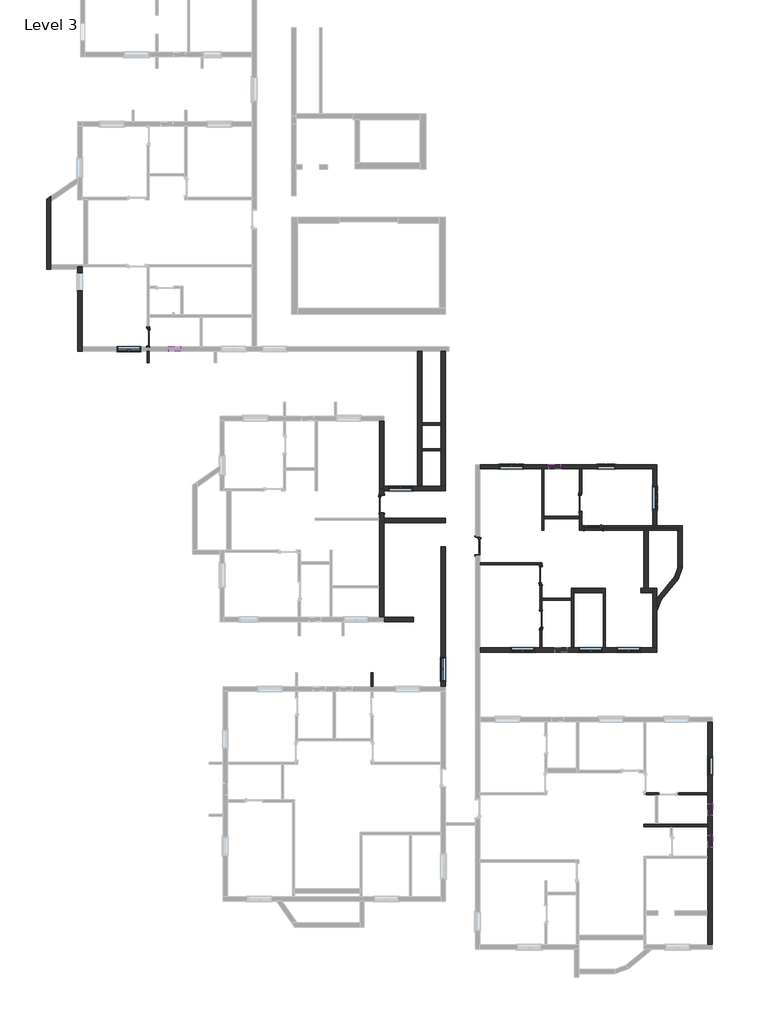
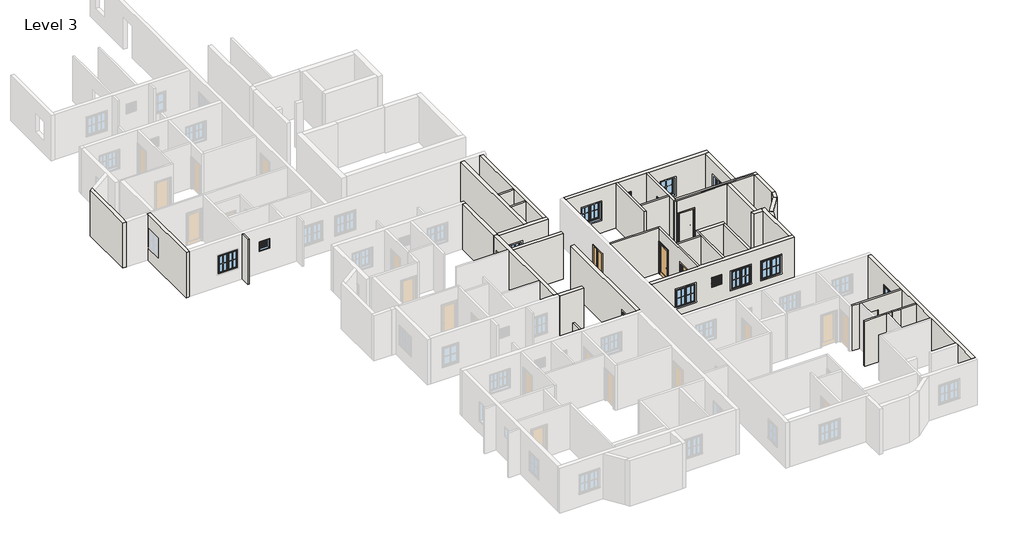
# One storey, part 3 of 7: 39 walls, 15 windows, 7 doors.
"""IFC4 building model written with IfcOpenShell, lengths in millimetres."""

from ifc_helpers import new_model, si_unit, point, frame, frame_2d, origin, place, context, project, spatial, polyline, circle_curve, trimmed, segment, composite_curve, outline, extrude, faceted_brep, transform, mapped, element, save
from components import door_3c6ab76a, door_a3feeac7, door_3b97b8e7, door_868ee8a9, window_272f20d6, window_casement_double_4_x_4_af3140d2, window_f2d8fef0

model = new_model("IFC4")

# Units and contexts
model_context = context("Model", 3, world=origin())
ifc_project = project(units=[si_unit("LENGTHUNIT", "METRE", prefix="MILLI")], contexts=[model_context])

# Site, building, storey
site = spatial("IfcSite", under=ifc_project)
building = spatial("IfcBuilding", under=site)
storey = spatial("IfcBuildingStorey", under=building, Name="Level 3", Elevation=3200.4)

# Doors
placement = place(None, origin())
door_shape = door_3c6ab76a(model_context)
element("IfcDoor", 1, ObjectType="Door-Interior-Single-1_Panel-Wood : 2'6\" x 7' door", at=placement, inside=storey, context=model_context, shape_type="MappedRepresentation", body=[
    mapped(door_shape, transform((-11252.4759469, 2064.0461172, 3200.4), x_axis=(0.0, -1.0, 0.0), y_axis=(1.0, 0.0, 0.0), z_axis=(0.0, 0.0, 1.0))),
])
door_2_shape = door_a3feeac7(model_context)
element("IfcDoor", 2, ObjectType="Door-Interior-Single-1_Panel-Wood : 2'6\" x 7' door", at=placement, inside=storey, context=model_context, shape_type="MappedRepresentation", body=[
    mapped(door_2_shape, transform((11042.3740531, -6465.2997229, 3200.4), x_axis=(0.0, -1.0, 0.0), y_axis=(1.0, 0.0, 0.0), z_axis=(0.0, 0.0, 1.0))),
])
element("IfcDoor", 3, ObjectType="Door-Interior-Single-1_Panel-Wood : 2'6\" x 7' door", at=placement, inside=storey, context=model_context, shape_type="MappedRepresentation", body=[
    mapped(door_2_shape, transform((9004.0240531, -12510.4997229, 3200.4), x_axis=(0.0, 1.0, 0.0), y_axis=(-1.0, 0.0, 0.0), z_axis=(0.0, 0.0, 1.0))),
])
element("IfcDoor", 4, ObjectType="Door-Interior-Single-1_Panel-Wood : 36\" x 84\"", at=placement, inside=storey, context=model_context, shape_type="MappedRepresentation", body=[
    mapped(door_shape, transform((8997.6740531, -10224.4997229, 3200.4), x_axis=(0.0, 1.0, 0.0), y_axis=(-1.0, 0.0, 0.0), z_axis=(0.0, 0.0, 1.0))),
])
door_3_shape = door_3b97b8e7(model_context)
element("IfcDoor", 5, ObjectType="Door-Interior-Single-1_Panel-Wood : 36\" x 84\"", at=placement, inside=storey, context=model_context, shape_type="MappedRepresentation", body=[
    mapped(door_3_shape, transform((5733.7740531, -8700.4997229, 3200.4), x_axis=(0.0, -1.0, 0.0), y_axis=(1.0, 0.0, 0.0), z_axis=(0.0, 0.0, 1.0))),
])
door_4_shape = door_868ee8a9(model_context)
element("IfcDoor", 6, ObjectType="Door-Interior-Single-1_Panel-Wood : 36\" x 84\"", at=placement, inside=storey, context=model_context, shape_type="MappedRepresentation", body=[
    mapped(door_4_shape, transform((787.1240531, -6537.0288828, 3200.4), x_axis=(0.0, -1.0, 0.0), y_axis=(1.0, 0.0, 0.0), z_axis=(0.0, 0.0, 1.0))),
])
element("IfcDoor", 7, ObjectType="Door-Interior-Single-1_Panel-Wood : 36\" x 84\"", at=placement, inside=storey, context=model_context, shape_type="MappedRepresentation", body=[
    mapped(door_4_shape, transform((11712.2990531, -7776.5747229, 3200.4), x_axis=(-1.0, 0.0, 0.0), y_axis=(0.0, -1.0, 0.0), z_axis=(0.0, 0.0, 1.0))),
])

# Walls
element("IfcWall", 8, ObjectType="4.5\" wall", at=placement, inside=storey, context=model_context, shape_type="SweptSolid", body=[
    extrude(outline(polyline([(-11312.8009469, 730.5461172), (-11312.8009469, 1340.1461172), (-11198.5009469, 1340.1461172), (-11198.5009469, 730.5461172), (-11312.8009469, 730.5461172)])), frame((0.0, 0.0, 3200.4), z_axis=(0.0, 0.0, 1.0), x_axis=(1.0, 0.0, 0.0)), (0.0, 0.0, 1.0), 3048.0),
])
element("IfcWall", 9, ObjectType="4.5\" wall", at=placement, inside=storey, context=model_context, shape_type="SweptSolid", body=[
    extrude(outline(polyline([(3850.9990531, -3803.3538828), (2860.3990531, -3803.3538828), (2860.3990531, -3689.0538828), (3850.9990531, -3689.0538828), (3850.9990531, -3803.3538828)])), frame((0.0, 0.0, 3200.4), z_axis=(0.0, 0.0, 1.0), x_axis=(1.0, 0.0, 0.0)), (0.0, 0.0, 1.0), 3048.0),
])
element("IfcWall", 10, ObjectType="4.5\" wall", at=placement, inside=storey, context=model_context, shape_type="SweptSolid", body=[
    extrude(outline(polyline([(2860.3990531, -2355.5538828), (3850.9990531, -2355.5538828), (3850.9990531, -2469.8538828), (2860.3990531, -2469.8538828), (2860.3990531, -2355.5538828)])), frame((0.0, 0.0, 3200.4), z_axis=(0.0, 0.0, 1.0), x_axis=(1.0, 0.0, 0.0)), (0.0, 0.0, 1.0), 3048.0),
])
element("IfcWall", 11, ObjectType="4.5\" wall", at=placement, inside=storey, context=model_context, shape_type="SweptSolid", body=[
    extrude(outline(polyline([(345.7990531, -15233.3538828), (345.7990531, -15957.2538828), (231.4990531, -15957.2538828), (231.4990531, -15233.3538828), (345.7990531, -15233.3538828)])), frame((0.0, 0.0, 3200.4), z_axis=(0.0, 0.0, 1.0), x_axis=(1.0, 0.0, 0.0)), (0.0, 0.0, 1.0), 3048.0),
])
element("IfcWall", 12, ObjectType="4.5\" wall", at=placement, inside=storey, context=model_context, shape_type="Brep", body=[
    faceted_brep([(17617.7990531, -21521.1497229, 6248.4), (15026.9990531, -21521.1497229, 6248.4), (14912.6990531, -21521.1497229, 6248.4), (14417.3990531, -21521.1497229, 6248.4), (14417.3990531, -21521.1497229, 3200.4), (14912.6990531, -21521.1497229, 3200.4), (15026.9990531, -21521.1497229, 3200.4), (15096.8490531, -21521.1497229, 3200.4), (15096.8490531, -21521.1497229, 5359.4), (16062.0490531, -21521.1497229, 5359.4), (16062.0490531, -21521.1497229, 3200.4), (17617.7990531, -21521.1497229, 3200.4), (14417.3990531, -21406.8497229, 6248.4), (17617.7990531, -21406.8497229, 6248.4), (17617.7990531, -21406.8497229, 3200.4), (16062.0490531, -21406.8497229, 3200.4), (16062.0490531, -21406.8497229, 5359.4), (15096.8490531, -21406.8497229, 5359.4), (15096.8490531, -21406.8497229, 3200.4), (14417.3990531, -21406.8497229, 3200.4)], [[[0, 1, 2, 3, 4, 5, 6, 7, 8, 9, 10, 11]], [[12, 13, 14, 15, 16, 17, 18, 19]], [[14, 11, 10, 15]], [[4, 19, 18, 7, 6, 5]], [[3, 2, 1, 0, 13, 12]], [[0, 11, 14, 13]], [[4, 3, 12, 19]], [[17, 8, 7, 18]], [[8, 17, 16, 9]], [[9, 16, 15, 10]]]),
])
element("IfcWall", 13, ObjectType="4.5\" wall", at=placement, inside=storey, context=model_context, shape_type="SweptSolid", body=[
    extrude(outline(polyline([(16055.6990531, -23045.1497229), (16589.0990531, -23045.1497229), (16589.0990531, -23159.4497229), (16055.6990531, -23159.4497229), (16055.6990531, -23045.1497229)])), frame((0.0, 0.0, 3200.4), z_axis=(0.0, 0.0, 1.0), x_axis=(1.0, 0.0, 0.0)), (0.0, 0.0, 1.0), 3048.0),
])
element("IfcWall", 14, ObjectType="4.5\" wall", at=placement, inside=storey, context=model_context, shape_type="Brep", body=[
    faceted_brep([(17617.7990531, -23045.1497229, 3200.4), (15026.9990531, -23045.1497229, 3200.4), (14912.6990531, -23045.1497229, 3200.4), (14303.0990531, -23045.1497229, 3200.4), (14303.0990531, -23045.1497229, 6248.4), (14912.6990531, -23045.1497229, 6248.4), (15026.9990531, -23045.1497229, 6248.4), (17617.7990531, -23045.1497229, 6248.4), (17617.7990531, -23159.4497229, 3200.4), (17617.7990531, -23159.4497229, 6248.4), (15788.9990531, -23159.4497229, 6248.4), (15674.6990531, -23159.4497229, 6248.4), (14303.0990531, -23159.4497229, 6248.4), (14303.0990531, -23159.4497229, 3200.4), (15674.6990531, -23159.4497229, 3200.4), (15788.9990531, -23159.4497229, 3200.4)], [[[0, 1, 2, 3, 4, 5, 6, 7]], [[8, 9, 10, 11, 12, 13, 14, 15]], [[3, 2, 1, 0, 8, 15, 14, 13]], [[4, 3, 13, 12]], [[7, 6, 5, 4, 12, 11, 10, 9]], [[0, 7, 9, 8]]]),
])
element("IfcWall", 15, ObjectType="4.5\" wall", at=placement, inside=storey, context=model_context, shape_type="Brep", body=[
    faceted_brep([(10988.3990531, -7894.0497229, 3200.4), (14303.0990531, -7894.0497229, 3200.4), (14531.6990531, -7894.0497229, 3200.4), (16055.6990531, -7894.0497229, 3200.4), (16055.6990531, -7894.0497229, 6248.4), (14531.6990531, -7894.0497229, 6248.4), (14303.0990531, -7894.0497229, 6248.4), (10988.3990531, -7894.0497229, 6248.4), (10988.3990531, -7779.7497229, 3200.4), (10988.3990531, -7779.7497229, 6248.4), (11102.6990531, -7779.7497229, 6248.4), (14760.2990531, -7779.7497229, 6248.4), (14988.8990531, -7779.7497229, 6248.4), (16055.6990531, -7779.7497229, 6248.4), (16055.6990531, -7779.7497229, 3200.4), (14988.8990531, -7779.7497229, 3200.4), (14760.2990531, -7779.7497229, 3200.4), (11102.6990531, -7779.7497229, 3200.4)], [[[0, 1, 2, 3, 4, 5, 6, 7]], [[8, 9, 10, 11, 12, 13, 14, 15, 16, 17]], [[3, 2, 1, 0, 8, 17, 16, 15, 14]], [[7, 6, 5, 4, 13, 12, 11, 10, 9]], [[0, 7, 9, 8]], [[4, 3, 14, 13]]]),
])
element("IfcWall", 16, ObjectType="4.5\" wall", at=placement, inside=storey, context=model_context, shape_type="Brep", body=[
    faceted_brep([(10696.2990531, -13939.2497229, 3200.4), (10696.2990531, -11119.8497229, 3200.4), (10696.2990531, -10891.2497229, 3200.4), (10696.2990531, -10891.2497229, 6248.4), (10696.2990531, -11119.8497229, 6248.4), (10696.2990531, -13939.2497229, 6248.4), (10581.9990531, -13939.2497229, 3200.4), (10581.9990531, -13939.2497229, 6248.4), (10581.9990531, -11500.8497229, 6248.4), (10581.9990531, -11386.5497229, 6248.4), (10581.9990531, -10891.2497229, 6248.4), (10581.9990531, -10891.2497229, 3200.4), (10581.9990531, -11386.5497229, 3200.4), (10581.9990531, -11500.8497229, 3200.4)], [[[0, 1, 2, 3, 4, 5]], [[6, 7, 8, 9, 10, 11, 12, 13]], [[2, 1, 0, 6, 13, 12, 11]], [[5, 4, 3, 10, 9, 8, 7]], [[0, 5, 7, 6]], [[3, 2, 11, 10]]]),
])
element("IfcWall", 17, ObjectType="4.5\" wall", at=placement, inside=storey, context=model_context, shape_type="SweptSolid", body=[
    extrude(outline(polyline([(9057.9990531, -11386.5497229), (10581.9990531, -11386.5497229), (10581.9990531, -11500.8497229), (9057.9990531, -11500.8497229), (9057.9990531, -11386.5497229)])), frame((0.0, 0.0, 3200.4), z_axis=(0.0, 0.0, 1.0), x_axis=(1.0, 0.0, 0.0)), (0.0, 0.0, 1.0), 3048.0),
])
element("IfcWall", 18, ObjectType="4.5\" wall", at=placement, inside=storey, context=model_context, shape_type="Brep", body=[
    faceted_brep([(8943.6990531, -13939.2497229, 6248.4), (8943.6990531, -9672.0497229, 6248.4), (8943.6990531, -9557.7497229, 6248.4), (8943.6990531, -9557.7497229, 3200.4), (8943.6990531, -9672.0497229, 3200.4), (8943.6990531, -9741.8997229, 3200.4), (8943.6990531, -9741.8997229, 5359.4), (8943.6990531, -10707.0997229, 5359.4), (8943.6990531, -10707.0997229, 3200.4), (8943.6990531, -12027.8997229, 3200.4), (8943.6990531, -12027.8997229, 5359.4), (8943.6990531, -12993.0997229, 5359.4), (8943.6990531, -12993.0997229, 3200.4), (8943.6990531, -13939.2497229, 3200.4), (9057.9990531, -9557.7497229, 6248.4), (9057.9990531, -11386.5497229, 6248.4), (9057.9990531, -11500.8497229, 6248.4), (9057.9990531, -13939.2497229, 6248.4), (9057.9990531, -13939.2497229, 3200.4), (9057.9990531, -12993.0997229, 3200.4), (9057.9990531, -12993.0997229, 5359.4), (9057.9990531, -12027.8997229, 5359.4), (9057.9990531, -12027.8997229, 3200.4), (9057.9990531, -11500.8497229, 3200.4), (9057.9990531, -11386.5497229, 3200.4), (9057.9990531, -10707.0997229, 3200.4), (9057.9990531, -10707.0997229, 5359.4), (9057.9990531, -9741.8997229, 5359.4), (9057.9990531, -9741.8997229, 3200.4), (9057.9990531, -9557.7497229, 3200.4)], [[[0, 1, 2, 3, 4, 5, 6, 7, 8, 9, 10, 11, 12, 13]], [[14, 15, 16, 17, 18, 19, 20, 21, 22, 23, 24, 25, 26, 27, 28, 29]], [[18, 13, 12, 19]], [[3, 29, 28, 5, 4]], [[22, 9, 8, 25, 24, 23]], [[2, 1, 0, 17, 16, 15, 14]], [[0, 13, 18, 17]], [[3, 2, 14, 29]], [[21, 10, 9, 22]], [[10, 21, 20, 11]], [[11, 20, 19, 12]], [[27, 6, 5, 28]], [[6, 27, 26, 7]], [[7, 26, 25, 8]]]),
])
element("IfcWall", 19, ObjectType="4.5\" wall", at=placement, inside=storey, context=model_context, shape_type="SweptSolid", body=[
    extrude(outline(polyline([(8943.6990531, -9672.0497229), (5844.8990531, -9672.0497229), (5844.8990531, -9557.7497229), (8943.6990531, -9557.7497229), (8943.6990531, -9672.0497229)])), frame((0.0, 0.0, 3200.4), z_axis=(0.0, 0.0, 1.0), x_axis=(1.0, 0.0, 0.0)), (0.0, 0.0, 1.0), 3048.0),
])
element("IfcWall", 20, ObjectType="4.5\" wall", at=placement, inside=storey, context=model_context, shape_type="Brep", body=[
    faceted_brep([(9045.2990531, -4731.7497229, 3200.4), (9045.2990531, -7894.0497229, 3200.4), (9045.2990531, -7894.0497229, 6248.4), (9045.2990531, -4731.7497229, 6248.4), (9159.5990531, -4731.7497229, 3200.4), (9159.5990531, -4731.7497229, 6248.4), (9159.5990531, -7170.1497229, 6248.4), (9159.5990531, -7284.4497229, 6248.4), (9159.5990531, -7894.0497229, 6248.4), (9159.5990531, -7894.0497229, 3200.4), (9159.5990531, -7284.4497229, 3200.4), (9159.5990531, -7170.1497229, 3200.4)], [[[0, 1, 2, 3]], [[4, 5, 6, 7, 8, 9, 10, 11]], [[1, 0, 4, 11, 10, 9]], [[2, 1, 9, 8]], [[3, 2, 8, 7, 6, 5]], [[0, 3, 5, 4]]]),
])
element("IfcWall", 21, ObjectType="4.5\" wall", at=placement, inside=storey, context=model_context, shape_type="Brep", body=[
    faceted_brep([(10988.3990531, -7779.7497229, 6248.4), (10988.3990531, -7284.4497229, 6248.4), (10988.3990531, -7170.1497229, 6248.4), (10988.3990531, -4731.7497229, 6248.4), (10988.3990531, -4731.7497229, 3200.4), (10988.3990531, -5982.6997229, 3200.4), (10988.3990531, -5982.6997229, 5359.4), (10988.3990531, -6947.8997229, 5359.4), (10988.3990531, -6947.8997229, 3200.4), (10988.3990531, -7170.1497229, 3200.4), (10988.3990531, -7284.4497229, 3200.4), (10988.3990531, -7779.7497229, 3200.4), (11102.6990531, -4731.7497229, 6248.4), (11102.6990531, -7665.4497229, 6248.4), (11102.6990531, -7779.7497229, 6248.4), (11102.6990531, -7779.7497229, 3200.4), (11102.6990531, -7665.4497229, 3200.4), (11102.6990531, -6947.8997229, 3200.4), (11102.6990531, -6947.8997229, 5359.4), (11102.6990531, -5982.6997229, 5359.4), (11102.6990531, -5982.6997229, 3200.4), (11102.6990531, -4731.7497229, 3200.4)], [[[0, 1, 2, 3, 4, 5, 6, 7, 8, 9, 10, 11]], [[12, 13, 14, 15, 16, 17, 18, 19, 20, 21]], [[4, 21, 20, 5]], [[15, 11, 10, 9, 8, 17, 16]], [[3, 2, 1, 0, 14, 13, 12]], [[4, 3, 12, 21]], [[0, 11, 15, 14]], [[7, 18, 17, 8]], [[18, 7, 6, 19]], [[19, 6, 5, 20]]]),
])
element("IfcWall", 22, ObjectType="4.5\" wall", at=placement, inside=storey, context=model_context, shape_type="SweptSolid", body=[
    extrude(outline(polyline([(10988.3990531, -7284.4497229), (9159.5990531, -7284.4497229), (9159.5990531, -7170.1497229), (10988.3990531, -7170.1497229), (10988.3990531, -7284.4497229)])), frame((0.0, 0.0, 3200.4), z_axis=(0.0, 0.0, 1.0), x_axis=(1.0, 0.0, 0.0)), (0.0, 0.0, 1.0), 3048.0),
])
element("IfcWall", 23, ObjectType="4.5\" wall", at=placement, inside=storey, context=model_context, shape_type="SweptSolid", body=[
    extrude(outline(polyline([(12220.2990531, -13939.2497229), (12220.2990531, -11119.8497229), (12334.5990531, -11119.8497229), (12334.5990531, -13939.2497229), (12220.2990531, -13939.2497229)])), frame((0.0, 0.0, 3200.4), z_axis=(0.0, 0.0, 1.0), x_axis=(1.0, 0.0, 0.0)), (0.0, 0.0, 1.0), 3048.0),
])
element("IfcWall", 24, ObjectType="9\"", at=placement, inside=storey, context=model_context, shape_type="Brep", body=[
    faceted_brep([(-14894.2009469, 5683.5461172, 3200.4), (-14894.2009469, 5569.2461172, 3200.4), (-14894.2009469, 1340.1461172, 3200.4), (-14894.2009469, 1340.1461172, 6248.4), (-14894.2009469, 5569.2461172, 6248.4), (-14894.2009469, 5683.5461172, 6248.4), (-14894.2009469, 5378.7461172, 5334.0), (-14894.2009469, 4464.3461172, 5334.0), (-14894.2009469, 4464.3461172, 4114.8), (-14894.2009469, 5378.7461172, 4114.8), (-14665.6009469, 5683.5461172, 3200.4), (-14665.6009469, 5683.5461172, 6248.4), (-14665.6009469, 1568.7461172, 6248.4), (-14665.6009469, 1340.1461172, 6248.4), (-14665.6009469, 1340.1461172, 3200.4), (-14665.6009469, 1568.7461172, 3200.4), (-14665.6009469, 5378.7461172, 5334.0), (-14665.6009469, 5378.7461172, 4114.8), (-14665.6009469, 4464.3461172, 4114.8), (-14665.6009469, 4464.3461172, 5334.0)], [[[0, 1, 2, 3, 4, 5], [6, 7, 8, 9]], [[10, 11, 12, 13, 14, 15], [16, 17, 18, 19]], [[2, 1, 0, 10, 15, 14]], [[5, 4, 3, 13, 12, 11]], [[3, 2, 14, 13]], [[0, 5, 11, 10]], [[17, 16, 6, 9]], [[18, 17, 9, 8]], [[19, 18, 8, 7]], [[16, 19, 7, 6]]]),
])
element("IfcWall", 25, ObjectType="9\"", at=placement, inside=storey, context=model_context, shape_type="Brep", body=[
    faceted_brep([(904.5990531, -5746.4538828, 3200.4), (904.5990531, -5632.1538828, 3200.4), (904.5990531, -2241.2538828, 3200.4), (904.5990531, -2241.2538828, 6248.4), (904.5990531, -5632.1538828, 6248.4), (904.5990531, -5746.4538828, 6248.4), (675.9990531, -5746.4538828, 3200.4), (675.9990531, -5746.4538828, 6248.4), (675.9990531, -2241.2538828, 6248.4), (675.9990531, -2241.2538828, 3200.4)], [[[0, 1, 2, 3, 4, 5]], [[6, 7, 8, 9]], [[2, 1, 0, 6, 9]], [[5, 4, 3, 8, 7]], [[0, 5, 7, 6]], [[3, 2, 9, 8]]]),
])
element("IfcWall", 26, ObjectType="9\"", at=placement, inside=storey, context=model_context, shape_type="Brep", body=[
    faceted_brep([(904.5990531, -5746.4538828, 3200.4), (904.5990531, -5746.4538828, 6248.4), (904.5990531, -5860.7538828, 6248.4), (904.5990531, -7270.4538828, 6248.4), (904.5990531, -7499.0538828, 6248.4), (904.5990531, -12375.8538828, 6248.4), (904.5990531, -12375.8538828, 3200.4), (904.5990531, -7499.0538828, 3200.4), (904.5990531, -7270.4538828, 3200.4), (904.5990531, -7019.6288828, 3200.4), (904.5990531, -7019.6288828, 5359.4), (904.5990531, -6054.4288828, 5359.4), (904.5990531, -6054.4288828, 3200.4), (904.5990531, -5860.7538828, 3200.4), (675.9990531, -5746.4538828, 6248.4), (675.9990531, -5746.4538828, 3200.4), (675.9990531, -6054.4288828, 3200.4), (675.9990531, -6054.4288828, 5359.4), (675.9990531, -7019.6288828, 5359.4), (675.9990531, -7019.6288828, 3200.4), (675.9990531, -7270.4538828, 3200.4), (675.9990531, -7384.7538828, 3200.4), (675.9990531, -10737.5538828, 3200.4), (675.9990531, -10851.8538828, 3200.4), (675.9990531, -12375.8538828, 3200.4), (675.9990531, -12375.8538828, 6248.4), (675.9990531, -10851.8538828, 6248.4), (675.9990531, -10737.5538828, 6248.4), (675.9990531, -7384.7538828, 6248.4), (675.9990531, -7270.4538828, 6248.4)], [[[0, 1, 2, 3, 4, 5, 6, 7, 8, 9, 10, 11, 12, 13]], [[14, 15, 16, 17, 18, 19, 20, 21, 22, 23, 24, 25, 26, 27, 28, 29]], [[6, 24, 23, 22, 21, 20, 19, 9, 8, 7]], [[15, 0, 13, 12, 16]], [[1, 0, 15, 14]], [[5, 4, 3, 2, 1, 14, 29, 28, 27, 26, 25]], [[6, 5, 25, 24]], [[18, 10, 9, 19]], [[10, 18, 17, 11]], [[11, 17, 16, 12]]]),
])
element("IfcWall", 27, ObjectType="9\"", at=placement, inside=storey, context=model_context, shape_type="SweptSolid", body=[
    extrude(outline(polyline([(904.5990531, -7270.4538828), (4079.5990531, -7270.4538828), (4079.5990531, -7499.0538828), (904.5990531, -7499.0538828), (904.5990531, -7270.4538828)])), frame((0.0, 0.0, 3200.4), z_axis=(0.0, 0.0, 1.0), x_axis=(1.0, 0.0, 0.0)), (0.0, 0.0, 1.0), 3048.0),
])
element("IfcWall", 28, ObjectType="9\"", at=placement, inside=storey, context=model_context, shape_type="Brep", body=[
    faceted_brep([(904.5990531, -5860.7538828, 3200.4), (4079.5990531, -5860.7538828, 3200.4), (4079.5990531, -5860.7538828, 6248.4), (904.5990531, -5860.7538828, 6248.4), (2377.7990531, -5860.7538828, 5334.0), (2377.7990531, -5860.7538828, 4114.8), (1158.5990531, -5860.7538828, 4114.8), (1158.5990531, -5860.7538828, 5334.0), (904.5990531, -5632.1538828, 3200.4), (904.5990531, -5632.1538828, 6248.4), (2631.7990531, -5632.1538828, 6248.4), (2860.3990531, -5632.1538828, 6248.4), (3850.9990531, -5632.1538828, 6248.4), (4079.5990531, -5632.1538828, 6248.4), (4079.5990531, -5632.1538828, 3200.4), (3850.9990531, -5632.1538828, 3200.4), (2860.3990531, -5632.1538828, 3200.4), (2631.7990531, -5632.1538828, 3200.4), (2377.7990531, -5632.1538828, 5334.0), (1158.5990531, -5632.1538828, 5334.0), (1158.5990531, -5632.1538828, 4114.8), (2377.7990531, -5632.1538828, 4114.8), (904.5990531, -5746.4538828, 3200.4), (904.5990531, -5746.4538828, 6248.4)], [[[0, 1, 2, 3], [4, 5, 6, 7]], [[8, 9, 10, 11, 12, 13, 14, 15, 16, 17], [18, 19, 20, 21]], [[1, 0, 22, 8, 17, 16, 15, 14]], [[3, 2, 13, 12, 11, 10, 9, 23]], [[0, 3, 23, 9, 8, 22]], [[2, 1, 14, 13]], [[5, 4, 18, 21]], [[6, 5, 21, 20]], [[7, 6, 20, 19]], [[4, 7, 19, 18]]]),
])
element("IfcWall", 29, ObjectType="9\"", at=placement, inside=storey, context=model_context, shape_type="Brep", body=[
    faceted_brep([(2631.7990531, 1340.1461172, 3200.4), (2631.7990531, -5632.1538828, 3200.4), (2631.7990531, -5632.1538828, 6248.4), (2631.7990531, 1340.1461172, 6248.4), (2860.3990531, 1340.1461172, 3200.4), (2860.3990531, 1340.1461172, 6248.4), (2860.3990531, -2355.5538828, 6248.4), (2860.3990531, -2469.8538828, 6248.4), (2860.3990531, -3689.0538828, 6248.4), (2860.3990531, -3803.3538828, 6248.4), (2860.3990531, -5632.1538828, 6248.4), (2860.3990531, -5632.1538828, 3200.4), (2860.3990531, -3803.3538828, 3200.4), (2860.3990531, -3689.0538828, 3200.4), (2860.3990531, -2469.8538828, 3200.4), (2860.3990531, -2355.5538828, 3200.4)], [[[0, 1, 2, 3]], [[4, 5, 6, 7, 8, 9, 10, 11, 12, 13, 14, 15]], [[1, 0, 4, 15, 14, 13, 12, 11]], [[3, 2, 10, 9, 8, 7, 6, 5]], [[0, 3, 5, 4]], [[2, 1, 11, 10]]]),
])
element("IfcWall", 30, ObjectType="9\"", at=placement, inside=storey, context=model_context, shape_type="Brep", body=[
    faceted_brep([(4079.5990531, -5632.1538828, 3200.4), (4079.5990531, 1340.1461172, 3200.4), (4079.5990531, 1340.1461172, 6248.4), (4079.5990531, -5632.1538828, 6248.4), (3850.9990531, -5632.1538828, 3200.4), (3850.9990531, -5632.1538828, 6248.4), (3850.9990531, -3803.3538828, 6248.4), (3850.9990531, -3689.0538828, 6248.4), (3850.9990531, -2469.8538828, 6248.4), (3850.9990531, -2355.5538828, 6248.4), (3850.9990531, 1340.1461172, 6248.4), (3850.9990531, 1340.1461172, 3200.4), (3850.9990531, -2355.5538828, 3200.4), (3850.9990531, -2469.8538828, 3200.4), (3850.9990531, -3689.0538828, 3200.4), (3850.9990531, -3803.3538828, 3200.4)], [[[0, 1, 2, 3]], [[4, 5, 6, 7, 8, 9, 10, 11, 12, 13, 14, 15]], [[1, 0, 4, 15, 14, 13, 12, 11]], [[3, 2, 10, 9, 8, 7, 6, 5]], [[2, 1, 11, 10]], [[0, 3, 5, 4]]]),
])
element("IfcWall", 31, ObjectType="9\"", at=placement, inside=storey, context=model_context, shape_type="SweptSolid", body=[
    extrude(outline(polyline([(904.5990531, -12375.8538828), (2441.2990531, -12375.8538828), (2441.2990531, -12604.4538828), (904.5990531, -12604.4538828), (904.5990531, -12375.8538828)])), frame((0.0, 0.0, 3200.4), z_axis=(0.0, 0.0, 1.0), x_axis=(1.0, 0.0, 0.0)), (0.0, 0.0, 1.0), 3048.0),
])
element("IfcWall", 32, ObjectType="9\"", at=placement, inside=storey, context=model_context, shape_type="Brep", body=[
    faceted_brep([(17617.7990531, -17749.2497229, 3200.4), (17617.7990531, -21406.8497229, 3200.4), (17617.7990531, -21521.1497229, 3200.4), (17617.7990531, -23045.1497229, 3200.4), (17617.7990531, -23159.4497229, 3200.4), (17617.7990531, -24683.4497229, 3200.4), (17617.7990531, -24797.7497229, 3200.4), (17617.7990531, -27502.8497229, 3200.4), (17617.7990531, -27731.4497229, 3200.4), (17617.7990531, -29255.4497229, 3200.4), (17617.7990531, -29255.4497229, 6248.4), (17617.7990531, -27731.4497229, 6248.4), (17617.7990531, -27502.8497229, 6248.4), (17617.7990531, -24797.7497229, 6248.4), (17617.7990531, -24683.4497229, 6248.4), (17617.7990531, -23159.4497229, 6248.4), (17617.7990531, -23045.1497229, 6248.4), (17617.7990531, -21521.1497229, 6248.4), (17617.7990531, -21406.8497229, 6248.4), (17617.7990531, -17749.2497229, 6248.4), (17617.7990531, -22587.9497229, 5334.0), (17617.7990531, -22587.9497229, 4724.4), (17617.7990531, -21978.3497229, 4724.4), (17617.7990531, -21978.3497229, 5334.0), (17617.7990531, -23616.6497229, 5334.0), (17617.7990531, -24226.2497229, 5334.0), (17617.7990531, -24226.2497229, 4724.4), (17617.7990531, -23616.6497229, 4724.4), (17617.7990531, -19584.3997229, 5334.0), (17617.7990531, -20498.7997229, 5334.0), (17617.7990531, -20498.7997229, 4114.8), (17617.7990531, -19584.3997229, 4114.8), (17846.3990531, -17749.2497229, 3200.4), (17846.3990531, -17749.2497229, 6248.4), (17846.3990531, -29255.4497229, 6248.4), (17846.3990531, -29255.4497229, 3200.4), (17846.3990531, -22587.9497229, 5334.0), (17846.3990531, -21978.3497229, 5334.0), (17846.3990531, -21978.3497229, 4724.4), (17846.3990531, -22587.9497229, 4724.4), (17846.3990531, -23616.6497229, 5334.0), (17846.3990531, -23616.6497229, 4724.4), (17846.3990531, -24226.2497229, 4724.4), (17846.3990531, -24226.2497229, 5334.0), (17846.3990531, -19584.3997229, 5334.0), (17846.3990531, -19584.3997229, 4114.8), (17846.3990531, -20498.7997229, 4114.8), (17846.3990531, -20498.7997229, 5334.0)], [[[0, 1, 2, 3, 4, 5, 6, 7, 8, 9, 10, 11, 12, 13, 14, 15, 16, 17, 18, 19], [20, 21, 22, 23], [24, 25, 26, 27], [28, 29, 30, 31]], [[32, 33, 34, 35], [36, 37, 38, 39], [40, 41, 42, 43], [44, 45, 46, 47]], [[9, 8, 7, 6, 5, 4, 3, 2, 1, 0, 32, 35]], [[19, 18, 17, 16, 15, 14, 13, 12, 11, 10, 34, 33]], [[0, 19, 33, 32]], [[10, 9, 35, 34]], [[21, 20, 36, 39]], [[22, 21, 39, 38]], [[23, 22, 38, 37]], [[20, 23, 37, 36]], [[41, 40, 24, 27]], [[42, 41, 27, 26]], [[43, 42, 26, 25]], [[40, 43, 25, 24]], [[45, 44, 28, 31]], [[46, 45, 31, 30]], [[47, 46, 30, 29]], [[44, 47, 29, 28]]]),
])
element("IfcWall", 33, ObjectType="9\"", at=placement, inside=storey, context=model_context, shape_type="Brep", body=[
    faceted_brep([(5844.8990531, -14167.8497229, 3200.4), (14988.8990531, -14167.8497229, 3200.4), (14988.8990531, -14167.8497229, 6248.4), (5844.8990531, -14167.8497229, 6248.4), (10334.3490531, -14167.8497229, 5334.0), (10334.3490531, -14167.8497229, 4724.4), (9724.7490531, -14167.8497229, 4724.4), (9724.7490531, -14167.8497229, 5334.0), (12912.4490531, -14167.8497229, 5334.0), (14131.6490531, -14167.8497229, 5334.0), (14131.6490531, -14167.8497229, 4114.8), (12912.4490531, -14167.8497229, 4114.8), (10956.6490531, -14167.8497229, 5334.0), (12175.8490531, -14167.8497229, 5334.0), (12175.8490531, -14167.8497229, 4114.8), (10956.6490531, -14167.8497229, 4114.8), (7451.4490531, -14167.8497229, 5334.0), (8670.6490531, -14167.8497229, 5334.0), (8670.6490531, -14167.8497229, 4114.8), (7451.4490531, -14167.8497229, 4114.8), (5844.8990531, -13939.2497229, 3200.4), (5844.8990531, -13939.2497229, 6248.4), (8943.6990531, -13939.2497229, 6248.4), (9057.9990531, -13939.2497229, 6248.4), (10581.9990531, -13939.2497229, 6248.4), (10696.2990531, -13939.2497229, 6248.4), (12220.2990531, -13939.2497229, 6248.4), (12334.5990531, -13939.2497229, 6248.4), (14760.2990531, -13939.2497229, 6248.4), (14988.8990531, -13939.2497229, 6248.4), (14988.8990531, -13939.2497229, 3200.4), (14760.2990531, -13939.2497229, 3200.4), (12334.5990531, -13939.2497229, 3200.4), (12220.2990531, -13939.2497229, 3200.4), (10696.2990531, -13939.2497229, 3200.4), (10581.9990531, -13939.2497229, 3200.4), (9057.9990531, -13939.2497229, 3200.4), (8943.6990531, -13939.2497229, 3200.4), (10334.3490531, -13939.2497229, 5334.0), (9724.7490531, -13939.2497229, 5334.0), (9724.7490531, -13939.2497229, 4724.4), (10334.3490531, -13939.2497229, 4724.4), (12912.4490531, -13939.2497229, 5334.0), (12912.4490531, -13939.2497229, 4114.8), (14131.6490531, -13939.2497229, 4114.8), (14131.6490531, -13939.2497229, 5334.0), (10956.6490531, -13939.2497229, 5334.0), (10956.6490531, -13939.2497229, 4114.8), (12175.8490531, -13939.2497229, 4114.8), (12175.8490531, -13939.2497229, 5334.0), (7451.4490531, -13939.2497229, 5334.0), (7451.4490531, -13939.2497229, 4114.8), (8670.6490531, -13939.2497229, 4114.8), (8670.6490531, -13939.2497229, 5334.0)], [[[0, 1, 2, 3], [4, 5, 6, 7], [8, 9, 10, 11], [12, 13, 14, 15], [16, 17, 18, 19]], [[20, 21, 22, 23, 24, 25, 26, 27, 28, 29, 30, 31, 32, 33, 34, 35, 36, 37], [38, 39, 40, 41], [42, 43, 44, 45], [46, 47, 48, 49], [50, 51, 52, 53]], [[1, 0, 20, 37, 36, 35, 34, 33, 32, 31, 30]], [[3, 2, 29, 28, 27, 26, 25, 24, 23, 22, 21]], [[0, 3, 21, 20]], [[2, 1, 30, 29]], [[5, 4, 38, 41]], [[6, 5, 41, 40]], [[7, 6, 40, 39]], [[4, 7, 39, 38]], [[43, 42, 8, 11]], [[44, 43, 11, 10]], [[45, 44, 10, 9]], [[42, 45, 9, 8]], [[47, 46, 12, 15]], [[48, 47, 15, 14]], [[49, 48, 14, 13]], [[46, 49, 13, 12]], [[51, 50, 16, 19]], [[52, 51, 19, 18]], [[53, 52, 18, 17]], [[50, 53, 17, 16]]]),
])
element("IfcWall", 34, ObjectType="9\"", at=placement, inside=storey, context=model_context, shape_type="SweptSolid", body=[
    extrude(outline(polyline([(-15957.2538828, 3200.4), (-15957.2538828, 6248.4), (-8732.9659091, 6248.4), (-8732.9659091, 3200.4), (-15957.2538828, 3200.4)]), holes=[polyline([(-14445.9538828, 5334.0), (-15665.1538828, 5334.0), (-15665.1538828, 4114.8), (-14445.9538828, 4114.8), (-14445.9538828, 5334.0)])]), frame((3850.9990531, 0.0, 0.0), z_axis=(1.0, 0.0, 0.0), x_axis=(0.0, 1.0, 0.0)), (0.0, 0.0, 1.0), 228.6),
])
element("IfcWall", 35, ObjectType="9\"", at=placement, inside=storey, context=model_context, shape_type="Brep", body=[
    faceted_brep([(5844.8990531, -4731.7497229, 3200.4), (9045.2990531, -4731.7497229, 3200.4), (9159.5990531, -4731.7497229, 3200.4), (10988.3990531, -4731.7497229, 3200.4), (11102.6990531, -4731.7497229, 3200.4), (14760.2990531, -4731.7497229, 3200.4), (14988.8990531, -4731.7497229, 3200.4), (14988.8990531, -4731.7497229, 6248.4), (14760.2990531, -4731.7497229, 6248.4), (11102.6990531, -4731.7497229, 6248.4), (10988.3990531, -4731.7497229, 6248.4), (9159.5990531, -4731.7497229, 6248.4), (9045.2990531, -4731.7497229, 6248.4), (5844.8990531, -4731.7497229, 6248.4), (10016.8490531, -4731.7497229, 5334.0), (10016.8490531, -4731.7497229, 4724.4), (9407.2490531, -4731.7497229, 4724.4), (9407.2490531, -4731.7497229, 5334.0), (12823.5490531, -4731.7497229, 5334.0), (12823.5490531, -4731.7497229, 4114.8), (11909.1490531, -4731.7497229, 4114.8), (11909.1490531, -4731.7497229, 5334.0), (8086.4490531, -4731.7497229, 5334.0), (8086.4490531, -4731.7497229, 4114.8), (6867.2490531, -4731.7497229, 4114.8), (6867.2490531, -4731.7497229, 5334.0), (5844.8990531, -4503.1497229, 3200.4), (5844.8990531, -4503.1497229, 6248.4), (14988.8990531, -4503.1497229, 6248.4), (14988.8990531, -4503.1497229, 3200.4), (10016.8490531, -4503.1497229, 5334.0), (9407.2490531, -4503.1497229, 5334.0), (9407.2490531, -4503.1497229, 4724.4), (10016.8490531, -4503.1497229, 4724.4), (12823.5490531, -4503.1497229, 5334.0), (11909.1490531, -4503.1497229, 5334.0), (11909.1490531, -4503.1497229, 4114.8), (12823.5490531, -4503.1497229, 4114.8), (8086.4490531, -4503.1497229, 5334.0), (6867.2490531, -4503.1497229, 5334.0), (6867.2490531, -4503.1497229, 4114.8), (8086.4490531, -4503.1497229, 4114.8)], [[[0, 1, 2, 3, 4, 5, 6, 7, 8, 9, 10, 11, 12, 13], [14, 15, 16, 17], [18, 19, 20, 21], [22, 23, 24, 25]], [[26, 27, 28, 29], [30, 31, 32, 33], [34, 35, 36, 37], [38, 39, 40, 41]], [[6, 5, 4, 3, 2, 1, 0, 26, 29]], [[13, 12, 11, 10, 9, 8, 7, 28, 27]], [[7, 6, 29, 28]], [[0, 13, 27, 26]], [[15, 14, 30, 33]], [[16, 15, 33, 32]], [[17, 16, 32, 31]], [[14, 17, 31, 30]], [[19, 18, 34, 37]], [[20, 19, 37, 36]], [[21, 20, 36, 35]], [[18, 21, 35, 34]], [[23, 22, 38, 41]], [[24, 23, 41, 40]], [[25, 24, 40, 39]], [[22, 25, 39, 38]]]),
])
element("IfcWall", 36, ObjectType="9\"", at=placement, inside=storey, context=model_context, shape_type="SweptSolid", body=[
    extrude(outline(polyline([(-7779.7497229, 3200.4), (-7779.7497229, 6248.4), (-4731.7497229, 6248.4), (-4731.7497229, 3200.4), (-7779.7497229, 3200.4)]), holes=[polyline([(-6836.7747229, 5334.0), (-6836.7747229, 4114.8), (-5617.5747229, 4114.8), (-5617.5747229, 5334.0), (-6836.7747229, 5334.0)])]), frame((14760.2990531, 0.0, 0.0), z_axis=(1.0, 0.0, 0.0), x_axis=(0.0, 1.0, 0.0)), (0.0, 0.0, 1.0), 228.6),
])
element("IfcWall", 37, ObjectType="9\"", at=placement, inside=storey, context=model_context, shape_type="Brep", body=[
    faceted_brep([(14988.8990531, -13939.2497229, 3200.4), (14988.8990531, -12059.0648255, 3200.4), (14988.8990531, -11373.2648255, 3200.4), (14988.8990531, -10891.2497229, 3200.4), (14988.8990531, -10891.2497229, 6248.4), (14988.8990531, -11373.2648255, 6248.4), (14988.8990531, -12059.0648255, 6248.4), (14988.8990531, -13939.2497229, 6248.4), (14760.2990531, -13939.2497229, 3200.4), (14760.2990531, -13939.2497229, 6248.4), (14760.2990531, -11119.8497229, 6248.4), (14760.2990531, -10891.2497229, 6248.4), (14760.2990531, -10891.2497229, 3200.4), (14760.2990531, -11119.8497229, 3200.4)], [[[0, 1, 2, 3, 4, 5, 6, 7]], [[8, 9, 10, 11, 12, 13]], [[3, 2, 1, 0, 8, 13, 12]], [[7, 6, 5, 4, 11, 10, 9]], [[0, 7, 9, 8]], [[4, 3, 12, 11]]]),
])
element("IfcWall", 38, ObjectType="9\"", at=placement, inside=storey, context=model_context, shape_type="SweptSolid", body=[
    extrude(outline(polyline([(14531.6990531, -7894.0497229), (14531.6990531, -10891.2497229), (14303.0990531, -10891.2497229), (14303.0990531, -7894.0497229), (14531.6990531, -7894.0497229)])), frame((0.0, 0.0, 3200.4), z_axis=(0.0, 0.0, 1.0), x_axis=(1.0, 0.0, 0.0)), (0.0, 0.0, 1.0), 3048.0),
])
element("IfcWall", 39, ObjectType="9\"", at=placement, inside=storey, context=model_context, shape_type="Brep", body=[
    faceted_brep([(10696.2990531, -11119.8497229, 3200.4), (12220.2990531, -11119.8497229, 3200.4), (12334.5990531, -11119.8497229, 3200.4), (12334.5990531, -11119.8497229, 6248.4), (12220.2990531, -11119.8497229, 6248.4), (10696.2990531, -11119.8497229, 6248.4), (10696.2990531, -10891.2497229, 3200.4), (10696.2990531, -10891.2497229, 6248.4), (12334.5990531, -10891.2497229, 6248.4), (12334.5990531, -10891.2497229, 3200.4)], [[[0, 1, 2, 3, 4, 5]], [[6, 7, 8, 9]], [[2, 1, 0, 6, 9]], [[5, 4, 3, 8, 7]], [[0, 5, 7, 6]], [[3, 2, 9, 8]]]),
])
element("IfcWall", 40, ObjectType="9\"", at=placement, inside=storey, context=model_context, shape_type="Brep", body=[
    faceted_brep([(14150.6990531, -11119.8497229, 3200.4), (14760.2990531, -11119.8497229, 3200.4), (14760.2990531, -11119.8497229, 6248.4), (14150.6990531, -11119.8497229, 6248.4), (14150.6990531, -10891.2497229, 3200.4), (14150.6990531, -10891.2497229, 6248.4), (14303.0990531, -10891.2497229, 6248.4), (14531.6990531, -10891.2497229, 6248.4), (14760.2990531, -10891.2497229, 6248.4), (14760.2990531, -10891.2497229, 3200.4), (14531.6990531, -10891.2497229, 3200.4), (14303.0990531, -10891.2497229, 3200.4)], [[[0, 1, 2, 3]], [[4, 5, 6, 7, 8, 9, 10, 11]], [[1, 0, 4, 11, 10, 9]], [[3, 2, 8, 7, 6, 5]], [[0, 3, 5, 4]], [[2, 1, 9, 8]]]),
])
element("IfcWall", 41, ObjectType="9\"", at=placement, inside=storey, context=model_context, shape_type="Brep", body=[
    faceted_brep([(-16265.8009469, 5569.2461172, 3200.4), (-16265.8009469, 5797.8461172, 3200.4), (-16265.8009469, 9043.9661172, 3200.4), (-16265.8009469, 9323.0079786, 3200.4), (-16265.8009469, 9323.0079786, 6248.4), (-16265.8009469, 9043.9661172, 6248.4), (-16265.8009469, 5797.8461172, 6248.4), (-16265.8009469, 5569.2461172, 6248.4), (-16494.4009469, 5569.2461172, 3200.4), (-16494.4009469, 5569.2461172, 6248.4), (-16494.4009469, 9162.9879786, 6248.4), (-16494.4009469, 9162.9879786, 3200.4)], [[[0, 1, 2, 3, 4, 5, 6, 7]], [[8, 9, 10, 11]], [[3, 2, 1, 0, 8, 11]], [[7, 6, 5, 4, 10, 9]], [[4, 3, 11, 10]], [[0, 7, 9, 8]]]),
])
element("IfcWall", 42, ObjectType="9\"", at=placement, inside=storey, context=model_context, shape_type="Brep", body=[
    faceted_brep([(16284.2990531, -7894.0497229, 6248.4), (16055.6990531, -7894.0497229, 6248.4), (11102.6990531, -7894.0497229, 6248.4), (11102.6990531, -7894.0497229, 3200.4), (11229.6990531, -7894.0497229, 3200.4), (11229.6990531, -7894.0497229, 5359.4), (12194.8990531, -7894.0497229, 5359.4), (12194.8990531, -7894.0497229, 3200.4), (16055.6990531, -7894.0497229, 3200.4), (16284.2990531, -7894.0497229, 3200.4), (11102.6990531, -7665.4497229, 6248.4), (16284.2990531, -7665.4497229, 6248.4), (16284.2990531, -7665.4497229, 3200.4), (12194.8990531, -7665.4497229, 3200.4), (12194.8990531, -7665.4497229, 5359.4), (11229.6990531, -7665.4497229, 5359.4), (11229.6990531, -7665.4497229, 3200.4), (11102.6990531, -7665.4497229, 3200.4), (11102.6990531, -7779.7497229, 3200.4), (11102.6990531, -7779.7497229, 6248.4)], [[[0, 1, 2, 3, 4, 5, 6, 7, 8, 9]], [[10, 11, 12, 13, 14, 15, 16, 17]], [[3, 18, 17, 16, 4]], [[12, 9, 8, 7, 13]], [[2, 1, 0, 11, 10, 19]], [[3, 2, 19, 10, 17, 18]], [[0, 9, 12, 11]], [[15, 5, 4, 16]], [[5, 15, 14, 6]], [[6, 14, 13, 7]]]),
])
element("IfcWall", 43, ObjectType="9\"", at=placement, inside=storey, context=model_context, shape_type="SweptSolid", body=[
    extrude(outline(polyline([(16055.6990531, -9831.602777), (16055.6990531, -7894.0497229), (16284.2990531, -7894.0497229), (16284.2990531, -9831.602777), (16055.6990531, -9831.602777)])), frame((0.0, 0.0, 3200.4), z_axis=(0.0, 0.0, 1.0), x_axis=(1.0, 0.0, 0.0)), (0.0, 0.0, 1.0), 3048.0),
])
element("IfcWall", 44, ObjectType="9\"", at=placement, inside=storey, context=model_context, shape_type="SweptSolid", body=[
    extrude(outline(polyline([(16075.314258, -10413.4246987), (15197.8838481, -11477.2429037), (15021.5300469, -11331.7874233), (15898.9604568, -10267.9692183), (16075.314258, -10413.4246987)])), frame((0.0, 0.0, 3200.4), z_axis=(0.0, 0.0, 1.0), x_axis=(1.0, 0.0, 0.0)), (0.0, 0.0, 1.0), 3048.0),
])
element("IfcWall", 45, ObjectType="9\"", at=placement, inside=storey, context=model_context, shape_type="SweptSolid", body=[
    extrude(outline(composite_curve([segment(polyline([(16055.6990531, -9831.602777), (16284.2990531, -9831.602777)]), True, "CONTINUOUS"), segment(trimmed(circle_curve(frame_2d((15369.8990531, -9831.602777)), 914.4), [point((16284.2990531, -9831.602777))], [point((16075.314258, -10413.4246987))], False, "CARTESIAN"), True, "CONTINUOUS"), segment(polyline([(16075.314258, -10413.4246987), (15898.9604568, -10267.9692183)]), True, "CONTINUOUS"), segment(trimmed(circle_curve(frame_2d((15369.8990531, -9831.602777)), 685.8), [point((15898.9604568, -10267.9692183))], [point((16055.6990531, -9831.602777))], True, "CARTESIAN"), True, "CONTINUOUS")], self_intersect=False)), frame((0.0, 0.0, 3200.4), z_axis=(0.0, 0.0, 1.0), x_axis=(1.0, 0.0, 0.0)), (0.0, 0.0, 1.0), 3048.0),
])
element("IfcWall", 46, ObjectType="9\"", at=placement, inside=storey, context=model_context, shape_type="SweptSolid", body=[
    extrude(outline(composite_curve([segment(trimmed(circle_curve(frame_2d((-12059.0648255, 15903.2990531)), 1143.0), [point((-11331.7874233, 15021.5300469))], [point((-11373.2648255, 14988.8990531))], False, "CARTESIAN"), True, "CONTINUOUS"), segment(polyline([(-11373.2648255, 14988.8990531), (-12059.0648255, 14988.8990531)]), True, "CONTINUOUS"), segment(trimmed(circle_curve(frame_2d((-12059.0648255, 15903.2990531)), 914.4), [point((-12059.0648255, 14988.8990531))], [point((-11477.2429037, 15197.8838481))], True, "CARTESIAN"), True, "CONTINUOUS"), segment(polyline([(-11477.2429037, 15197.8838481), (-11331.7874233, 15021.5300469)]), True, "CONTINUOUS")], self_intersect=False)), frame((0.0, 0.0, 6248.4), z_axis=(0.0, 0.0, -1.0), x_axis=(0.0, 1.0, 0.0)), (0.0, 0.0, 1.0), 3048.0),
])

# Windows
window_shape = window_272f20d6(model_context)
element("IfcWindow", 47, ObjectType="Window-Awning-Single : 36\" x 48\"", at=placement, inside=storey, context=model_context, shape_type="MappedRepresentation", body=[
    mapped(window_shape, transform((12366.3490531, -4617.4497229, 3200.4), x_axis=(1.0, 0.0, 0.0), y_axis=(0.0, 1.0, 0.0), z_axis=(0.0, 0.0, 1.0))),
])
element("IfcWindow", 48, ObjectType="Window-Awning-Single : 36\" x 48\"", at=placement, inside=storey, context=model_context, shape_type="MappedRepresentation", body=[
    mapped(window_shape, transform((17732.0990531, -20041.5997229, 3200.4), x_axis=(0.0, 1.0, 0.0), y_axis=(-1.0, 0.0, 0.0), z_axis=(0.0, 0.0, 1.0))),
])
window_casement_double_4_x_4_shape = window_casement_double_4_x_4_af3140d2(model_context)
element("IfcWindow", 49, ObjectType="Window-Casement-Double : 4' x 4'", at=placement, inside=storey, context=model_context, shape_type="MappedRepresentation", body=[
    mapped(window_casement_double_4_x_4_shape, transform((14874.5990531, -6227.1747229, 3200.4), x_axis=(0.0, -1.0, 0.0), y_axis=(1.0, 0.0, 0.0), z_axis=(0.0, 0.0, 1.0))),
])
element("IfcWindow", 50, ObjectType="Window-Casement-Double : 4' x 4'", at=placement, inside=storey, context=model_context, shape_type="MappedRepresentation", body=[
    mapped(window_casement_double_4_x_4_shape, transform((7476.8490531, -4617.4497229, 3200.4), x_axis=(1.0, 0.0, 0.0), y_axis=(0.0, 1.0, 0.0), z_axis=(0.0, 0.0, 1.0))),
])
element("IfcWindow", 51, ObjectType="Window-Casement-Double : 4' x 4'", at=placement, inside=storey, context=model_context, shape_type="MappedRepresentation", body=[
    mapped(window_casement_double_4_x_4_shape, transform((13522.0490531, -14053.5497229, 3200.4), x_axis=(-1.0, 0.0, 0.0), y_axis=(0.0, -1.0, 0.0), z_axis=(0.0, 0.0, 1.0))),
])
element("IfcWindow", 52, ObjectType="Window-Casement-Double : 4' x 4'", at=placement, inside=storey, context=model_context, shape_type="MappedRepresentation", body=[
    mapped(window_casement_double_4_x_4_shape, transform((11566.2490531, -14053.5497229, 3200.4), x_axis=(-1.0, 0.0, 0.0), y_axis=(0.0, -1.0, 0.0), z_axis=(0.0, 0.0, 1.0))),
])
element("IfcWindow", 53, ObjectType="Window-Casement-Double : 4' x 4'", at=placement, inside=storey, context=model_context, shape_type="MappedRepresentation", body=[
    mapped(window_casement_double_4_x_4_shape, transform((8061.0490531, -14053.5497229, 3200.4), x_axis=(-1.0, 0.0, 0.0), y_axis=(0.0, -1.0, 0.0), z_axis=(0.0, 0.0, 1.0))),
])
element("IfcWindow", 54, ObjectType="Window-Casement-Double : 4' x 4'", at=placement, inside=storey, context=model_context, shape_type="MappedRepresentation", body=[
    mapped(window_casement_double_4_x_4_shape, transform((3965.2990531, -15055.5538828, 3200.4), x_axis=(0.0, 1.0, 0.0), y_axis=(-1.0, 0.0, 0.0), z_axis=(0.0, 0.0, 1.0))),
])
element("IfcWindow", 55, ObjectType="Window-Casement-Double : 4' x 4'", at=placement, inside=storey, context=model_context, shape_type="MappedRepresentation", body=[
    mapped(window_casement_double_4_x_4_shape, transform((1768.1990531, -5746.4538828, 3200.4), x_axis=(1.0, 0.0, 0.0), y_axis=(0.0, 1.0, 0.0), z_axis=(0.0, 0.0, 1.0))),
])
element("IfcWindow", 56, ObjectType="Window-Casement-Double : 4' x 4'", at=placement, inside=storey, context=model_context, shape_type="MappedRepresentation", body=[
    mapped(window_casement_double_4_x_4_shape, transform((-12246.2509469, 1454.4461172, 3200.4), x_axis=(-1.0, 0.0, 0.0), y_axis=(0.0, -1.0, 0.0), z_axis=(0.0, 0.0, 1.0))),
])
window_2_shape = window_f2d8fef0(model_context)
element("IfcWindow", 57, ObjectType="Window-Louvers : 24\" x 24\"", at=placement, inside=storey, context=model_context, shape_type="MappedRepresentation", body=[
    mapped(window_2_shape, transform((-9890.4009469, 1460.7961172, 3810.0), x_axis=(1.0, 0.0, 0.0), y_axis=(0.0, 1.0, 0.0), z_axis=(0.0, 0.0, 1.0))),
])
element("IfcWindow", 58, ObjectType="Window-Louvers : 24\" x 24\"", at=placement, inside=storey, context=model_context, shape_type="MappedRepresentation", body=[
    mapped(window_2_shape, transform((9712.0490531, -4623.7997229, 3810.0), x_axis=(-1.0, 0.0, 0.0), y_axis=(0.0, -1.0, 0.0), z_axis=(0.0, 0.0, 1.0))),
])
element("IfcWindow", 59, ObjectType="Window-Louvers : 24\" x 24\"", at=placement, inside=storey, context=model_context, shape_type="MappedRepresentation", body=[
    mapped(window_2_shape, transform((10029.5490531, -14059.8997229, 3810.0), x_axis=(-1.0, 0.0, 0.0), y_axis=(0.0, -1.0, 0.0), z_axis=(0.0, 0.0, 1.0))),
])
element("IfcWindow", 60, ObjectType="Window-Louvers : 24\" x 24\"", at=placement, inside=storey, context=model_context, shape_type="MappedRepresentation", body=[
    mapped(window_2_shape, transform((17725.7490531, -22283.1497229, 3810.0), x_axis=(0.0, 1.0, 0.0), y_axis=(-1.0, 0.0, 0.0), z_axis=(0.0, 0.0, 1.0))),
])
element("IfcWindow", 61, ObjectType="Window-Louvers : 24\" x 24\"", at=placement, inside=storey, context=model_context, shape_type="MappedRepresentation", body=[
    mapped(window_2_shape, transform((17738.4490531, -23921.4497229, 3810.0), x_axis=(0.0, -1.0, 0.0), y_axis=(1.0, 0.0, 0.0), z_axis=(0.0, 0.0, 1.0))),
])

save(model, "model.ifc")

# Revit data of these elements
# Type "Door-Interior-Single-1_Panel-Wood : 2'6\" x 7' door"
#   Type Mark = "9"
#   Assembly Code = "C1020300"
#   Analytic Construction = "Wooden"
#   Top Rail = 0' - 4 11/16"
#   Thickness = 0' - 1 3/8"
#   Thermal Resistance (R) = 2.5876 (h·ft²·°F)/BTU
#   Swing Angle [instance default] = 90.00°
#   Stiles = 0' - 4 3/4"
#   Rough Width = 3' - 2"
#   Rough Height = 7' - 1"
#   Height = 7' - 0"
#   Width = 3' - 0"
#   Heat Transfer Coefficient (U) = 0.3865 BTU/(h·ft²·°F)
#   Bottom Rail = 0' - 9 1/8"
#   Trim Material = Cherry
#   Panel Material = Cherry
#   Frame Material = Cherry
#   Door Handle Material = Aluminum
#   Visual Light Transmittance = 0
#   Solar Heat Gain Coefficient = 0
#   Wall Closure = (empty or 0)
#   Function = (empty or 0)
# Type "Door-Interior-Single-1_Panel-Wood : 36\" x 84\""
#   Type Mark = "8"
#   Assembly Code = "C1020300"
#   Analytic Construction = "Wooden"
#   Top Rail = 0' - 4 11/16"
#   Thickness = 0' - 1 3/8"
#   Thermal Resistance (R) = 2.5876 (h·ft²·°F)/BTU
#   Swing Angle [instance default] = 90.00°
#   Stiles = 0' - 4 3/4"
#   Rough Width = 3' - 2"
#   Rough Height = 7' - 1"
#   Height = 7' - 0"
#   Width = 3' - 0"
#   Heat Transfer Coefficient (U) = 0.3865 BTU/(h·ft²·°F)
#   Bottom Rail = 0' - 9 1/8"
#   Trim Material = Cherry
#   Panel Material = Cherry
#   Frame Material = Cherry
#   Door Handle Material = Aluminum
#   Visual Light Transmittance = 0
#   Solar Heat Gain Coefficient = 0
#   Wall Closure = (empty or 0)
#   Function = (empty or 0)
# Type "4.5\" wall"
#   Assembly Code = "B2010"
#   Layers, outside or top first: 0' - 4 1/2" no material (function 1)
# Type "9\""
#   Assembly Code = "B2010"
#   Layers, outside or top first: 0' - 9" no material (function 1)
# Type "Window-Awning-Single : 36\" x 48\""
#   Type Mark = "20"
#   Fire Rating = "0.5h"
#   Assembly Code = "B2020100"
#   Analytic Construction = "Double glazing - domestic"
#   Window Inset [instance default] = 0' - 0"
#   Wall Thickness [instance default] = 0' - 6"
#   Visual Light Transmittance = 0.81
#   Thermal Resistance (R) = 1.8146 (h·ft²·°F)/BTU
#   Solar Heat Gain Coefficient = 0.76
#   Rough Width = 3' - 0 1/2"
#   Rough Height = 4' - 0 1/2"
#   Interior Wall Closure [instance default] = 0' - 2 1/4"
#   Height = 4' - 0"
#   Heat Transfer Coefficient (U) = 0.5511 BTU/(h·ft²·°F)
#   Frame Extension [instance default] = 0' - 0 1/4"
#   Exterior Wall Closure [instance default] = 0' - 1 1/4"
#   Extension Jamb [instance default] = 0' - 2 1/4"
#   Default Sill Height = 3' - 0"
#   Width = 3' - 0"
#   Muntin Visibility = yes
#   Interior Trim Visibility [instance default] = yes
#   Exterior Trim Visibility [instance default] = yes
#   Extension Jamb Visibility [instance default] = yes
#   Muntin Pattern = Muntin Pattern_2x2 : Muntin Pattern_2x2
#   Interior Trim Material = Wood - Stained
#   Interior Trim = Trim-Window-Interior-Flat : Picture Frame
#   Interior Frame Material = Wood - Stained
#   Glass Panel Material = Glass
#   Exterior Trim Material = Clad - White
#   Exterior Trim = Trim-Window-Exterior-Flat : with Sill
#   Exterior Frame Material = Clad - White
#   Wall Closure = (empty or 0)
# Type "Window-Casement-Double : 4' x 4'"
#   Type Mark = "21"
#   Fire Rating = "0.5h"
#   Assembly Code = "B2020100"
#   Analytic Construction = "Double glazing - domestic"
#   Frame Extension [instance default] = 0' - 0 1/4"
#   Window Inset [instance default] = 0' - 0"
#   Wall Thickness [instance default] = 0' - 6"
#   Interior Wall Closure [instance default] = 0' - 2 1/4"
#   Half Width = 2' - 0"
#   Visual Light Transmittance = 0.81
#   Thermal Resistance (R) = 1.8146 (h·ft²·°F)/BTU
#   Solar Heat Gain Coefficient = 0.76
#   Rough Width = 4' - 0 1/2"
#   Rough Height = 4' - 0 1/2"
#   Height = 4' - 0"
#   Heat Transfer Coefficient (U) = 0.5511 BTU/(h·ft²·°F)
#   Exterior Wall Closure [instance default] = 0' - 1 1/4"
#   Extension Jamb [instance default] = 0' - 2 1/4"
#   Default Sill Height = 3' - 0"
#   Width = 4' - 0"
#   Muntin Visibility = yes
#   Interior Trim Visibility [instance default] = yes
#   Exterior Trim Visibility [instance default] = yes
#   Extension Jamb Visibility [instance default] = yes
#   Interior Trim Material = Wood - Stained
#   Muntin Pattern = Muntin Pattern_2x2 : Muntin Pattern_2x2
#   Interior Trim = Trim-Window-Interior-Flat : Picture Frame
#   Interior Frame Material = Wood - Stained
#   Glass Panel Material = Glass
#   Exterior Trim Material = Clad - White
#   Exterior Trim = Trim-Window-Exterior-Flat : with Sill
#   Exterior Frame Material = Clad - White
#   Wall Closure = (empty or 0)
# Type "Window-Louvers : 24\" x 24\""
#   Type Mark = "18"
#   Construction Type Id = "GSP4R"
#   Assembly Code = "B20"
#   Analytic Construction = "1/8 in Pilkington single glazing"
#   Visual Light Transmittance = 0.9
#   Thermal Resistance (R) = 1.53941 (h·ft²·°F)/BTU
#   Solar Heat Gain Coefficient = 0.78
#   Max Height = 1' - 11.74264"
#   Height = 2' - 0"
#   Heat Transfer Coefficient (U) = 0.6496 BTU/(h·ft²·°F)
#   Blade Width [instance default] = 1' - 10 1/2"
#   Blade Vertical Thickness = 0' - 0.35355"
#   Blade Thickness = 0' - 0 1/4"
#   Blade Spacing = 0' - 1 1/2"
#   Blade Height = 0' - 1.85355"
#   Blade Depth = 0' - 3"
#   Blade Angle = 45.00°
#   Default Sill Height = 3' - 0"
#   Trim Projection_Exterior = 0' - 0 1/2"
#   Trim Projection_Interior = 0' - 0 1/2"
#   Trim Width_Exterior = 0' - 1 1/2"
#   Trim Width_Interior = 0' - 1 1/2"
#   Width = 2' - 0"
#   Max Blade Count = 12
#   Define Thermal Properties by = 1
#   Blade Count = 12
#   Frame Material = Birch
#   Louver Material = Birch
#   Trim Exterior Material = Birch
#   Trim Interior Material = Birch
#   Wall Closure = (empty or 0)
# Elements 1, 2, 3 (IfcDoor, "Door-Interior-Single-1_Panel-Wood : 2'6\" x 7' door")
#   Swing Angle = 90.00°
#   Phase Created = New Construction
#   Materials on its faces: "Cherry", "Aluminum"
# Elements 4, 5, 6, 7 (IfcDoor, "Door-Interior-Single-1_Panel-Wood : 36\" x 84\"")
#   Swing Angle = 90.00°
#   Phase Created = New Construction
#   Materials on its faces: "Cherry", "Aluminum"
# Elements 8, 9, 10, 11, 12, 13, 14, 15, 16, 17, 18, 19, 20, 21, 22, 23 (IfcWall, "4.5\" wall")
#   Top Offset = 0' - 0"
#   Base Offset = 0' - 0"
#   wall height = 10' - 0"
#   Phase Created = New Construction
#   Base Constraint = Level 3
#   Top Constraint = Level 4
#   Materials on its faces: "Default Wall"
# Elements 24, 25, 26, 27, 28, 29, 30, 31, 32, 33, 34, 35, 36, 37, 38, 39, 40, 41, 42, 43, 44 (IfcWall, "9\"")
#   Top Offset = 0' - 0"
#   Base Offset = 0' - 0"
#   wall height = 10' - 0"
#   Phase Created = New Construction
#   Base Constraint = Level 3
#   Top Constraint = Level 4
#   Materials on its faces: "Default Wall"
# Elements 45, 46 (IfcWall, "9\"")
#   Top Offset = 0' - 0"
#   Base Offset = 0' - 0"
#   Unconnected Height = 20' - 0"
#   wall height = 10' - 0"
#   Phase Created = New Construction
#   Materials on its faces: "Default Wall"
# Element 47 (IfcWindow, "Window-Awning-Single : 36\" x 48\"")
#   Mark = "26"
#   Window Inset = 0' - 0"
#   Interior Wall Closure = 0' - 2 1/4"
#   Frame Extension = 0' - 0 1/4"
#   Exterior Wall Closure = 0' - 1 1/4"
#   Interior Trim Visibility = yes
#   Exterior Trim Visibility = yes
#   Phase Created = New Construction
#   Materials on its faces: "Wood - Stained", "Glass", "Clad - White"
# Element 48 (IfcWindow, "Window-Awning-Single : 36\" x 48\"")
#   Mark = "27"
#   Window Inset = 0' - 0"
#   Interior Wall Closure = 0' - 2 1/4"
#   Frame Extension = 0' - 0 1/4"
#   Exterior Wall Closure = 0' - 1 1/4"
#   Interior Trim Visibility = yes
#   Exterior Trim Visibility = yes
#   Phase Created = New Construction
#   Materials on its faces: "Wood - Stained", "Glass", "Clad - White"
# Element 49 (IfcWindow, "Window-Casement-Double : 4' x 4'")
#   Mark = "40"
#   Window Inset = 0' - 0"
#   Interior Wall Closure = 0' - 2 1/4"
#   Frame Extension = 0' - 0 1/4"
#   Exterior Wall Closure = 0' - 1 1/4"
#   Interior Trim Visibility = yes
#   Exterior Trim Visibility = yes
#   Phase Created = New Construction
#   Materials on its faces: "Wood - Stained", "Glass", "Clad - White"
# Element 50 (IfcWindow, "Window-Casement-Double : 4' x 4'")
#   Mark = "41"
#   Window Inset = 0' - 0"
#   Interior Wall Closure = 0' - 2 1/4"
#   Frame Extension = 0' - 0 1/4"
#   Exterior Wall Closure = 0' - 1 1/4"
#   Interior Trim Visibility = yes
#   Exterior Trim Visibility = yes
#   Phase Created = New Construction
#   Materials on its faces: "Wood - Stained", "Glass", "Clad - White"
# Element 51 (IfcWindow, "Window-Casement-Double : 4' x 4'")
#   Mark = "42"
#   Window Inset = 0' - 0"
#   Interior Wall Closure = 0' - 2 1/4"
#   Frame Extension = 0' - 0 1/4"
#   Exterior Wall Closure = 0' - 1 1/4"
#   Interior Trim Visibility = yes
#   Exterior Trim Visibility = yes
#   Phase Created = New Construction
#   Materials on its faces: "Wood - Stained", "Glass", "Clad - White"
# Element 52 (IfcWindow, "Window-Casement-Double : 4' x 4'")
#   Mark = "43"
#   Window Inset = 0' - 0"
#   Interior Wall Closure = 0' - 2 1/4"
#   Frame Extension = 0' - 0 1/4"
#   Exterior Wall Closure = 0' - 1 1/4"
#   Interior Trim Visibility = yes
#   Exterior Trim Visibility = yes
